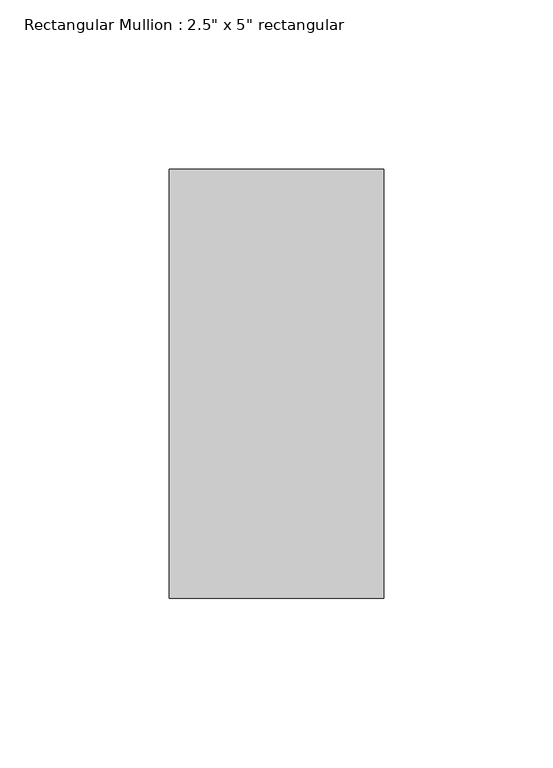
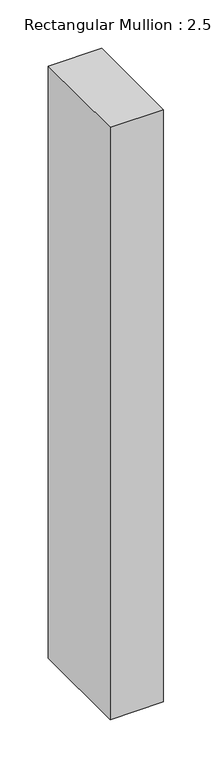
"""IFC4 building model written with IfcOpenShell, lengths in millimetres: member geometry."""

from ifc_helpers import new_model, si_unit, frame, origin, place, context, project, spatial, polyline, outline, extrude, source, transform, mapped, element, save


def member_da260789(model_context):
    return source(origin(), model_context, "Body", "SweptSolid", [
        extrude(outline(polyline([(0.0, 63.5), (0.0, -63.5), (-63.5, -63.5), (-63.5, 63.5), (0.0, 63.5)])), frame((0.0, 0.0, -745.5377103), z_axis=(0.0, 0.0, 1.0), x_axis=(1.0, 0.0, 0.0)), (0.0, 0.0, 1.0), 745.5377103),
    ])


if __name__ == "__main__":
    model = new_model("IFC4")
    model_context = context("Model", 3, world=origin())
    ifc_project = project(units=[si_unit("LENGTHUNIT", "METRE", prefix="MILLI")], contexts=[model_context])
    site = spatial("IfcSite", under=ifc_project)
    building = spatial("IfcBuilding", under=site)
    placement = place(None, origin())
    member_shape = member_da260789(model_context)
    element("IfcMember", 1, ObjectType="Rectangular Mullion : 2.5\" x 5\" rectangular", at=placement, inside=building, context=model_context, shape_type="MappedRepresentation", body=[
        mapped(member_shape, transform((0.0, 0.0, 0.0), x_axis=(1.0, 0.0, 0.0), y_axis=(0.0, 1.0, 0.0), z_axis=(0.0, 0.0, 1.0))),
    ])
    save(model, "model.ifc")

# Revit data of these elements
# Type "Rectangular Mullion : 2.5\" x 5\" rectangular"
#   built-in parameter 1007304 = 0.416667 (stored number, unit not read)
#   built-in parameter 1007301 = 0.104167 (stored number, unit not read)
#   built-in parameter 1007300 = 0.104167 (stored number, unit not read)
# Element 1 (IfcMember, "Rectangular Mullion : 2.5\" x 5\" rectangular")
#   Materials on its faces: "Aluminum"
# Materials
#   "Aluminum": class "Metal", colour RGB 247 247 247, transparency 0, Description = "Aluminum 6061", Cost = 0
